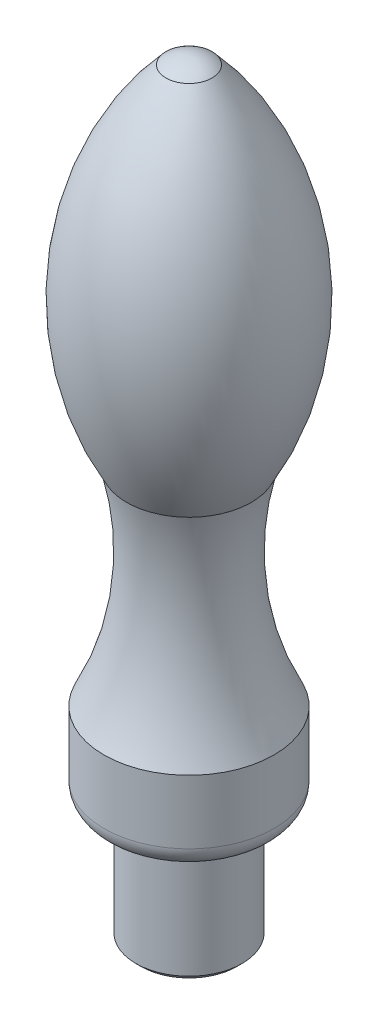
SolidWorks part; units mm, degrees
material "Plain Carbon Steel"
ref_plane "Front Plane" through (0, 0, 0) normal (0, 0, 1) x (1, 0, 0)
ref_plane "Top Plane" through (0, 0, 0) normal (0, 1, 0) x (1, 0, 0)
ref_plane "Right Plane" through (0, 0, 0) normal (1, 0, 0) x (0, 0, -1)
sketch "Shank Sketch Ø10" plane through (0, 0, 0) normal (0, 1, 0) x (1, 0, 0)
  circle A0 centre (0, 0) radius 5
  dimension "D1" = 10
extrude "Shank Ø10" add sketch "Shank Sketch Ø10" along normal blind 11
chamfer "Shank End Chamfer 0.5" distance 0.5 angle 45 1 edges at (0, 0, 5)
sketch "Collar Sketch Ø16" plane through (0, 11, 0) normal (0, 1, 0) x (1, 0, 0)
  circle A0 centre (0, 0) radius 8
  dimension "D1" = 16
extrude "Collar Ø16" add sketch "Collar Sketch Ø16" along normal blind 8
fillet "Collar Fillet R2" radius 2 1 edges at (0, 11, 8)
sketch "Grip Profile Sketch" plane through (0, 0, 0) normal (0, 0, 1) x (1, 0, 0)
  line L0 (0, 0) -> (0, 72) construction
  line L1 (-8, 19) -> (0, 19)
  line L2 (8, 19) -> (-8, 19) construction
  line L3 (0, 72) -> (0, 19)
  arc A0 (-8, 19) -> (-5.866, 38.5212) centre (-32.9997, 31.6101) ccw
  arc A1 (-5.866, 38.5212) -> (-2.1656, 71.2666) centre (18.4797, 52.3517) cw
  arc A5 (0, 72) -> (-2.1656, 71.2666) centre (0, 68.4361) ccw
  dimension "D2" = 72
  dimension "D3" = 3.5639
  dimension "D1" = 28
  dimension "D4" = 28
  dimension "D5" = 18.4797
  dimension "D6" = 2.1656
  dimension "D7" = 5.866
revolve "Grip Knob" add sketch "Grip Profile Sketch" angle 360 about L0
